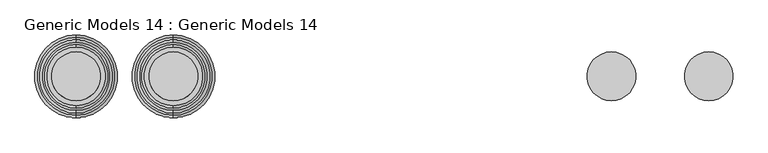
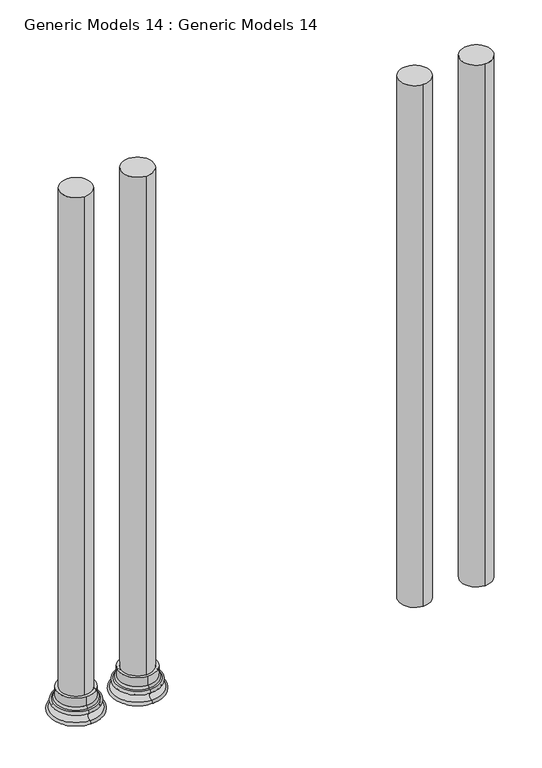
"""IFC4 building model written with IfcOpenShell, lengths in millimetres: proxy geometry, Generic Models 14 : Generic Models 14."""

from ifc_helpers import new_model, si_unit, point, frame, frame_2d, origin, place, context, project, spatial, polyline, circle_curve, ellipse_curve, trimmed, segment, composite_curve, outline, extrude, source, transform, mapped, element, save
from ifc_brep_helpers import plane_surface, cylinder_surface, revolved_surface, advanced_brep


def generic_models_14_generic_models_14_26f09abb(model_context):
    return source(origin(), model_context, "Body", "SolidModel", [
        advanced_brep(
        [(-2055.6825076, -7335.7292912, 330.2), (-2055.6825076, -7742.1292912, 330.2), (-2055.6825076, -7742.1292912, 304.8), (-2055.6825076, -7335.7292912, 304.8), (-2055.6825076, -7356.4126296, 381.908346), (-2055.6825076, -7721.4459527, 381.908346), (-2055.6825076, -7361.1292912, 406.4), (-2055.6825076, -7716.7292912, 406.4), (-2055.6825076, -7386.5292912, 431.8), (-2055.6825076, -7691.3292912, 431.8), (-2055.6825076, -7691.3292912, 406.4), (-2055.6825076, -7386.5292912, 406.4), (-2055.6825076, -7386.5292912, 508.0), (-2055.6825076, -7691.3292912, 508.0), (-2055.6825076, -7411.9292912, 304.8), (-2055.6825076, -7665.9292912, 304.8), (-2055.6825076, -7665.9292912, 508.0), (-2055.6825076, -7411.9292912, 508.0)],
        [
            (0, 1, circle_curve(frame((-2055.6825076, -7538.9292912, 330.2), z_axis=(0.0, 0.0, -1.0), x_axis=(0.0, -1.0, 0.0)), 203.2)),
            (1, 2, circle_curve(frame((-2055.6825076, -7742.1292912, 317.5), z_axis=(1.0, 0.0, 0.0), x_axis=(0.0, -1.0, 0.0)), 12.7)),
            (2, 3, circle_curve(frame((-2055.6825076, -7538.9292912, 304.8), z_axis=(0.0, 0.0, 1.0), x_axis=(0.0, -1.0, 0.0)), 203.2)),
            (3, 0, circle_curve(frame((-2055.6825076, -7335.7292912, 317.5), z_axis=(1.0, 0.0, 0.0), x_axis=(0.0, 1.0, 0.0)), 12.7)),
            (4, 5, circle_curve(frame((-2055.6825076, -7538.9292912, 381.908346), z_axis=(0.0, 0.0, -1.0), x_axis=(0.0, -1.0, 0.0)), 182.5166616)),
            (5, 1, circle_curve(frame((-2055.6825076, -7742.1292912, 360.1908407), z_axis=(-1.0, 0.0, 0.0), x_axis=(0.0, -1.0, 0.0)), 29.9908407)),
            (0, 4, circle_curve(frame((-2055.6825076, -7335.7292912, 360.1908407), z_axis=(-1.0, 0.0, 0.0), x_axis=(0.0, 1.0, 0.0)), 29.9908407)),
            (6, 7, circle_curve(frame((-2055.6825076, -7538.9292912, 406.4), z_axis=(0.0, 0.0, -1.0), x_axis=(0.0, -1.0, 0.0)), 177.8)),
            (7, 5, circle_curve(frame((-2055.6825076, -7716.7292912, 393.7), z_axis=(1.0, 0.0, 0.0), x_axis=(0.0, -1.0, 0.0)), 12.7)),
            (4, 6, circle_curve(frame((-2055.6825076, -7361.1292912, 393.7), z_axis=(1.0, 0.0, 0.0), x_axis=(0.0, 1.0, 0.0)), 12.7)),
            (8, 9, circle_curve(frame((-2055.6825076, -7538.9292912, 431.8), z_axis=(0.0, 0.0, -1.0), x_axis=(0.0, -1.0, 0.0)), 152.4)),
            (9, 10, circle_curve(frame((-2055.6825076, -7691.3292912, 419.1), z_axis=(1.0, 0.0, 0.0), x_axis=(0.0, -1.0, 0.0)), 12.7)),
            (10, 11, circle_curve(frame((-2055.6825076, -7538.9292912, 406.4), z_axis=(0.0, 0.0, 1.0), x_axis=(0.0, -1.0, 0.0)), 152.4)),
            (11, 8, circle_curve(frame((-2055.6825076, -7386.5292912, 419.1), z_axis=(1.0, 0.0, 0.0), x_axis=(0.0, 1.0, 0.0)), 12.7)),
            (12, 13, circle_curve(frame((-2055.6825076, -7538.9292912, 508.0), z_axis=(0.0, 0.0, -1.0), x_axis=(0.0, -1.0, 0.0)), 152.4)),
            (13, 9),
            (8, 12),
            (14, 15, circle_curve(frame((-2055.6825076, -7538.9292912, 304.8), z_axis=(0.0, 0.0, -1.0), x_axis=(0.0, -1.0, 0.0)), 127.0)),
            (15, 16),
            (16, 17, circle_curve(frame((-2055.6825076, -7538.9292912, 508.0), z_axis=(0.0, 0.0, 1.0), x_axis=(0.0, -1.0, 0.0)), 127.0)),
            (17, 14),
            (1, 0, circle_curve(frame((-2055.6825076, -7538.9292912, 330.2), z_axis=(0.0, 0.0, -1.0), x_axis=(0.0, 1.0, 0.0)), 203.2)),
            (3, 2, circle_curve(frame((-2055.6825076, -7538.9292912, 304.8), z_axis=(0.0, 0.0, 1.0), x_axis=(0.0, 1.0, 0.0)), 203.2)),
            (5, 4, circle_curve(frame((-2055.6825076, -7538.9292912, 381.908346), z_axis=(0.0, 0.0, -1.0), x_axis=(0.0, 1.0, 0.0)), 182.5166616)),
            (7, 6, circle_curve(frame((-2055.6825076, -7538.9292912, 406.4), z_axis=(0.0, 0.0, -1.0), x_axis=(0.0, 1.0, 0.0)), 177.8)),
            (10, 11, circle_curve(frame((-2055.6825076, -7538.9292912, 406.4), z_axis=(0.0, 0.0, -1.0), x_axis=(0.0, 1.0, 0.0)), 152.4)),
            (9, 8, circle_curve(frame((-2055.6825076, -7538.9292912, 431.8), z_axis=(0.0, 0.0, -1.0), x_axis=(0.0, 1.0, 0.0)), 152.4)),
            (13, 12, circle_curve(frame((-2055.6825076, -7538.9292912, 508.0), z_axis=(0.0, 0.0, -1.0), x_axis=(0.0, 1.0, 0.0)), 152.4)),
            (16, 17, circle_curve(frame((-2055.6825076, -7538.9292912, 508.0), z_axis=(0.0, 0.0, -1.0), x_axis=(0.0, 1.0, 0.0)), 127.0)),
            (15, 14, circle_curve(frame((-2055.6825076, -7538.9292912, 304.8), z_axis=(0.0, 0.0, -1.0), x_axis=(0.0, 1.0, 0.0)), 127.0)),
        ],
        [
            revolved_surface(trimmed(ellipse_curve(frame((-2055.6825076, -7742.1292912, 317.5), z_axis=(-1.0, 0.0, 0.0), x_axis=(0.0, -1.0, 0.0)), 12.7, 12.7), [point((-2055.6825076, -7742.1292912, 304.8))], [point((-2055.6825076, -7742.1292912, 330.2))], True, "CARTESIAN"), (-2055.6825076, -7538.9292912, 304.8), (0.0, 0.0, 1.0)),
            revolved_surface(trimmed(ellipse_curve(frame((-2055.6825076, -7742.1292912, 360.1908407), z_axis=(1.0, 0.0, 0.0), x_axis=(0.0, -1.0, 0.0)), 29.9908407, 29.9908407), [point((-2055.6825076, -7742.1292912, 330.2))], [point((-2055.6825076, -7721.4459527, 381.908346))], True, "CARTESIAN"), (-2055.6825076, -7538.9292912, 304.8), (0.0, 0.0, 1.0)),
            revolved_surface(trimmed(ellipse_curve(frame((-2055.6825076, -7716.7292912, 393.7), z_axis=(-1.0, 0.0, 0.0), x_axis=(0.0, -1.0, 0.0)), 12.7, 12.7), [point((-2055.6825076, -7721.4459527, 381.908346))], [point((-2055.6825076, -7716.7292912, 406.4))], True, "CARTESIAN"), (-2055.6825076, -7538.9292912, 304.8), (0.0, 0.0, 1.0)),
            revolved_surface(trimmed(ellipse_curve(frame((-2055.6825076, -7691.3292912, 419.1), z_axis=(-1.0, 0.0, 0.0), x_axis=(0.0, -1.0, 0.0)), 12.7, 12.7), [point((-2055.6825076, -7691.3292912, 406.4))], [point((-2055.6825076, -7691.3292912, 431.8))], True, "CARTESIAN"), (-2055.6825076, -7538.9292912, 304.8), (0.0, 0.0, 1.0)),
            cylinder_surface(frame((-2055.6825076, -7538.9292912, 304.8), z_axis=(0.0, 0.0, 1.0), x_axis=(0.0, -1.0, 0.0)), 152.4),
            revolved_surface(polyline([(-2055.6825076, -7665.9292912, 508.0), (-2055.6825076, -7665.9292912, 304.8)]), (-2055.6825076, -7538.9292912, 304.8), (0.0, 0.0, 1.0)),
            revolved_surface(trimmed(ellipse_curve(frame((-2055.6825076, -7335.7292912, 317.5), z_axis=(1.0, 0.0, 0.0), x_axis=(0.0, 1.0, 0.0)), 12.7, 12.7), [point((-2055.6825076, -7335.7292912, 304.8))], [point((-2055.6825076, -7335.7292912, 330.2))], True, "CARTESIAN"), (-2055.6825076, -7538.9292912, 304.8), (0.0, 0.0, 1.0)),
            revolved_surface(trimmed(ellipse_curve(frame((-2055.6825076, -7335.7292912, 360.1908407), z_axis=(-1.0, 0.0, 0.0), x_axis=(0.0, 1.0, 0.0)), 29.9908407, 29.9908407), [point((-2055.6825076, -7335.7292912, 330.2))], [point((-2055.6825076, -7356.4126296, 381.908346))], True, "CARTESIAN"), (-2055.6825076, -7538.9292912, 304.8), (0.0, 0.0, 1.0)),
            revolved_surface(trimmed(ellipse_curve(frame((-2055.6825076, -7361.1292912, 393.7), z_axis=(1.0, 0.0, 0.0), x_axis=(0.0, 1.0, 0.0)), 12.7, 12.7), [point((-2055.6825076, -7356.4126296, 381.908346))], [point((-2055.6825076, -7361.1292912, 406.4))], True, "CARTESIAN"), (-2055.6825076, -7538.9292912, 304.8), (0.0, 0.0, 1.0)),
            plane_surface(frame((-2055.6825076, -7538.9292912, 406.4), z_axis=(0.0, 0.0, 1.0), x_axis=(0.0, 1.0, 0.0))),
            revolved_surface(trimmed(ellipse_curve(frame((-2055.6825076, -7386.5292912, 419.1), z_axis=(1.0, 0.0, 0.0), x_axis=(0.0, 1.0, 0.0)), 12.7, 12.7), [point((-2055.6825076, -7386.5292912, 406.4))], [point((-2055.6825076, -7386.5292912, 431.8))], True, "CARTESIAN"), (-2055.6825076, -7538.9292912, 304.8), (0.0, 0.0, 1.0)),
            cylinder_surface(frame((-2055.6825076, -7538.9292912, 304.8), z_axis=(0.0, 0.0, 1.0), x_axis=(0.0, 1.0, 0.0)), 152.4),
            plane_surface(frame((-2055.6825076, -7538.9292912, 508.0), z_axis=(0.0, 0.0, 1.0), x_axis=(0.0, 1.0, 0.0))),
            revolved_surface(polyline([(-2055.6825076, -7411.9292912, 508.0), (-2055.6825076, -7411.9292912, 304.8)]), (-2055.6825076, -7538.9292912, 304.8), (0.0, 0.0, 1.0)),
            plane_surface(frame((-2055.6825076, -7538.9292912, 304.8), z_axis=(0.0, 0.0, -1.0), x_axis=(0.0, 1.0, 0.0))),
        ],
        [
            (0, [[1, 2, 3, 4]]),
            (1, [[5, 6, -1, 7]]),
            (2, [[8, 9, -5, 10]]),
            (3, [[11, 12, 13, 14]]),
            (4, [[15, 16, -11, 17]]),
            (5, [[18, 19, 20, 21]]),
            (6, [[22, -4, 23, -2]]),
            (7, [[24, -7, -22, -6]]),
            (8, [[25, -10, -24, -9]]),
            (9, [[-25, -8], [26, -13]]),
            (10, [[27, -14, -26, -12]]),
            (11, [[28, -17, -27, -16]]),
            (12, [[-28, -15], [29, -20]]),
            (13, [[30, -21, -29, -19]]),
            (14, [[-23, -3], [-30, -18]]),
        ],
    ),
        advanced_brep(
        [(-2563.6825076, -7335.7292912, 330.2), (-2563.6825076, -7742.1292912, 330.2), (-2563.6825076, -7742.1292912, 304.8), (-2563.6825076, -7335.7292912, 304.8), (-2563.6825076, -7356.4126296, 381.908346), (-2563.6825076, -7721.4459527, 381.908346), (-2563.6825076, -7361.1292912, 406.4), (-2563.6825076, -7716.7292912, 406.4), (-2563.6825076, -7386.5292912, 431.8), (-2563.6825076, -7691.3292912, 431.8), (-2563.6825076, -7691.3292912, 406.4), (-2563.6825076, -7386.5292912, 406.4), (-2563.6825076, -7386.5292912, 508.0), (-2563.6825076, -7691.3292912, 508.0), (-2563.6825076, -7411.9292912, 304.8), (-2563.6825076, -7665.9292912, 304.8), (-2563.6825076, -7665.9292912, 508.0), (-2563.6825076, -7411.9292912, 508.0)],
        [
            (0, 1, circle_curve(frame((-2563.6825076, -7538.9292912, 330.2), z_axis=(0.0, 0.0, -1.0), x_axis=(0.0, -1.0, 0.0)), 203.2)),
            (1, 2, circle_curve(frame((-2563.6825076, -7742.1292912, 317.5), z_axis=(1.0, 0.0, 0.0), x_axis=(0.0, -1.0, 0.0)), 12.7)),
            (2, 3, circle_curve(frame((-2563.6825076, -7538.9292912, 304.8), z_axis=(0.0, 0.0, 1.0), x_axis=(0.0, -1.0, 0.0)), 203.2)),
            (3, 0, circle_curve(frame((-2563.6825076, -7335.7292912, 317.5), z_axis=(1.0, 0.0, 0.0), x_axis=(0.0, 1.0, 0.0)), 12.7)),
            (4, 5, circle_curve(frame((-2563.6825076, -7538.9292912, 381.908346), z_axis=(0.0, 0.0, -1.0), x_axis=(0.0, -1.0, 0.0)), 182.5166616)),
            (5, 1, circle_curve(frame((-2563.6825076, -7742.1292912, 360.1908407), z_axis=(-1.0, 0.0, 0.0), x_axis=(0.0, -1.0, 0.0)), 29.9908407)),
            (0, 4, circle_curve(frame((-2563.6825076, -7335.7292912, 360.1908407), z_axis=(-1.0, 0.0, 0.0), x_axis=(0.0, 1.0, 0.0)), 29.9908407)),
            (6, 7, circle_curve(frame((-2563.6825076, -7538.9292912, 406.4), z_axis=(0.0, 0.0, -1.0), x_axis=(0.0, -1.0, 0.0)), 177.8)),
            (7, 5, circle_curve(frame((-2563.6825076, -7716.7292912, 393.7), z_axis=(1.0, 0.0, 0.0), x_axis=(0.0, -1.0, 0.0)), 12.7)),
            (4, 6, circle_curve(frame((-2563.6825076, -7361.1292912, 393.7), z_axis=(1.0, 0.0, 0.0), x_axis=(0.0, 1.0, 0.0)), 12.7)),
            (8, 9, circle_curve(frame((-2563.6825076, -7538.9292912, 431.8), z_axis=(0.0, 0.0, -1.0), x_axis=(0.0, -1.0, 0.0)), 152.4)),
            (9, 10, circle_curve(frame((-2563.6825076, -7691.3292912, 419.1), z_axis=(1.0, 0.0, 0.0), x_axis=(0.0, -1.0, 0.0)), 12.7)),
            (10, 11, circle_curve(frame((-2563.6825076, -7538.9292912, 406.4), z_axis=(0.0, 0.0, 1.0), x_axis=(0.0, -1.0, 0.0)), 152.4)),
            (11, 8, circle_curve(frame((-2563.6825076, -7386.5292912, 419.1), z_axis=(1.0, 0.0, 0.0), x_axis=(0.0, 1.0, 0.0)), 12.7)),
            (12, 13, circle_curve(frame((-2563.6825076, -7538.9292912, 508.0), z_axis=(0.0, 0.0, -1.0), x_axis=(0.0, -1.0, 0.0)), 152.4)),
            (13, 9),
            (8, 12),
            (14, 15, circle_curve(frame((-2563.6825076, -7538.9292912, 304.8), z_axis=(0.0, 0.0, -1.0), x_axis=(0.0, -1.0, 0.0)), 127.0)),
            (15, 16),
            (16, 17, circle_curve(frame((-2563.6825076, -7538.9292912, 508.0), z_axis=(0.0, 0.0, 1.0), x_axis=(0.0, -1.0, 0.0)), 127.0)),
            (17, 14),
            (1, 0, circle_curve(frame((-2563.6825076, -7538.9292912, 330.2), z_axis=(0.0, 0.0, -1.0), x_axis=(0.0, 1.0, 0.0)), 203.2)),
            (3, 2, circle_curve(frame((-2563.6825076, -7538.9292912, 304.8), z_axis=(0.0, 0.0, 1.0), x_axis=(0.0, 1.0, 0.0)), 203.2)),
            (5, 4, circle_curve(frame((-2563.6825076, -7538.9292912, 381.908346), z_axis=(0.0, 0.0, -1.0), x_axis=(0.0, 1.0, 0.0)), 182.5166616)),
            (7, 6, circle_curve(frame((-2563.6825076, -7538.9292912, 406.4), z_axis=(0.0, 0.0, -1.0), x_axis=(0.0, 1.0, 0.0)), 177.8)),
            (10, 11, circle_curve(frame((-2563.6825076, -7538.9292912, 406.4), z_axis=(0.0, 0.0, -1.0), x_axis=(0.0, 1.0, 0.0)), 152.4)),
            (9, 8, circle_curve(frame((-2563.6825076, -7538.9292912, 431.8), z_axis=(0.0, 0.0, -1.0), x_axis=(0.0, 1.0, 0.0)), 152.4)),
            (13, 12, circle_curve(frame((-2563.6825076, -7538.9292912, 508.0), z_axis=(0.0, 0.0, -1.0), x_axis=(0.0, 1.0, 0.0)), 152.4)),
            (16, 17, circle_curve(frame((-2563.6825076, -7538.9292912, 508.0), z_axis=(0.0, 0.0, -1.0), x_axis=(0.0, 1.0, 0.0)), 127.0)),
            (15, 14, circle_curve(frame((-2563.6825076, -7538.9292912, 304.8), z_axis=(0.0, 0.0, -1.0), x_axis=(0.0, 1.0, 0.0)), 127.0)),
        ],
        [
            revolved_surface(trimmed(ellipse_curve(frame((-2563.6825076, -7742.1292912, 317.5), z_axis=(-1.0, 0.0, 0.0), x_axis=(0.0, -1.0, 0.0)), 12.7, 12.7), [point((-2563.6825076, -7742.1292912, 304.8))], [point((-2563.6825076, -7742.1292912, 330.2))], True, "CARTESIAN"), (-2563.6825076, -7538.9292912, 304.8), (0.0, 0.0, 1.0)),
            revolved_surface(trimmed(ellipse_curve(frame((-2563.6825076, -7742.1292912, 360.1908407), z_axis=(1.0, 0.0, 0.0), x_axis=(0.0, -1.0, 0.0)), 29.9908407, 29.9908407), [point((-2563.6825076, -7742.1292912, 330.2))], [point((-2563.6825076, -7721.4459527, 381.908346))], True, "CARTESIAN"), (-2563.6825076, -7538.9292912, 304.8), (0.0, 0.0, 1.0)),
            revolved_surface(trimmed(ellipse_curve(frame((-2563.6825076, -7716.7292912, 393.7), z_axis=(-1.0, 0.0, 0.0), x_axis=(0.0, -1.0, 0.0)), 12.7, 12.7), [point((-2563.6825076, -7721.4459527, 381.908346))], [point((-2563.6825076, -7716.7292912, 406.4))], True, "CARTESIAN"), (-2563.6825076, -7538.9292912, 304.8), (0.0, 0.0, 1.0)),
            revolved_surface(trimmed(ellipse_curve(frame((-2563.6825076, -7691.3292912, 419.1), z_axis=(-1.0, 0.0, 0.0), x_axis=(0.0, -1.0, 0.0)), 12.7, 12.7), [point((-2563.6825076, -7691.3292912, 406.4))], [point((-2563.6825076, -7691.3292912, 431.8))], True, "CARTESIAN"), (-2563.6825076, -7538.9292912, 304.8), (0.0, 0.0, 1.0)),
            cylinder_surface(frame((-2563.6825076, -7538.9292912, 304.8), z_axis=(0.0, 0.0, 1.0), x_axis=(0.0, -1.0, 0.0)), 152.4),
            revolved_surface(polyline([(-2563.6825076, -7665.9292912, 508.0), (-2563.6825076, -7665.9292912, 304.8)]), (-2563.6825076, -7538.9292912, 304.8), (0.0, 0.0, 1.0)),
            revolved_surface(trimmed(ellipse_curve(frame((-2563.6825076, -7335.7292912, 317.5), z_axis=(1.0, 0.0, 0.0), x_axis=(0.0, 1.0, 0.0)), 12.7, 12.7), [point((-2563.6825076, -7335.7292912, 304.8))], [point((-2563.6825076, -7335.7292912, 330.2))], True, "CARTESIAN"), (-2563.6825076, -7538.9292912, 304.8), (0.0, 0.0, 1.0)),
            revolved_surface(trimmed(ellipse_curve(frame((-2563.6825076, -7335.7292912, 360.1908407), z_axis=(-1.0, 0.0, 0.0), x_axis=(0.0, 1.0, 0.0)), 29.9908407, 29.9908407), [point((-2563.6825076, -7335.7292912, 330.2))], [point((-2563.6825076, -7356.4126296, 381.908346))], True, "CARTESIAN"), (-2563.6825076, -7538.9292912, 304.8), (0.0, 0.0, 1.0)),
            revolved_surface(trimmed(ellipse_curve(frame((-2563.6825076, -7361.1292912, 393.7), z_axis=(1.0, 0.0, 0.0), x_axis=(0.0, 1.0, 0.0)), 12.7, 12.7), [point((-2563.6825076, -7356.4126296, 381.908346))], [point((-2563.6825076, -7361.1292912, 406.4))], True, "CARTESIAN"), (-2563.6825076, -7538.9292912, 304.8), (0.0, 0.0, 1.0)),
            plane_surface(frame((-2563.6825076, -7538.9292912, 406.4), z_axis=(0.0, 0.0, 1.0), x_axis=(0.0, 1.0, 0.0))),
            revolved_surface(trimmed(ellipse_curve(frame((-2563.6825076, -7386.5292912, 419.1), z_axis=(1.0, 0.0, 0.0), x_axis=(0.0, 1.0, 0.0)), 12.7, 12.7), [point((-2563.6825076, -7386.5292912, 406.4))], [point((-2563.6825076, -7386.5292912, 431.8))], True, "CARTESIAN"), (-2563.6825076, -7538.9292912, 304.8), (0.0, 0.0, 1.0)),
            cylinder_surface(frame((-2563.6825076, -7538.9292912, 304.8), z_axis=(0.0, 0.0, 1.0), x_axis=(0.0, 1.0, 0.0)), 152.4),
            plane_surface(frame((-2563.6825076, -7538.9292912, 508.0), z_axis=(0.0, 0.0, 1.0), x_axis=(0.0, 1.0, 0.0))),
            revolved_surface(polyline([(-2563.6825076, -7411.9292912, 508.0), (-2563.6825076, -7411.9292912, 304.8)]), (-2563.6825076, -7538.9292912, 304.8), (0.0, 0.0, 1.0)),
            plane_surface(frame((-2563.6825076, -7538.9292912, 304.8), z_axis=(0.0, 0.0, -1.0), x_axis=(0.0, 1.0, 0.0))),
        ],
        [
            (0, [[1, 2, 3, 4]]),
            (1, [[5, 6, -1, 7]]),
            (2, [[8, 9, -5, 10]]),
            (3, [[11, 12, 13, 14]]),
            (4, [[15, 16, -11, 17]]),
            (5, [[18, 19, 20, 21]]),
            (6, [[22, -4, 23, -2]]),
            (7, [[24, -7, -22, -6]]),
            (8, [[25, -10, -24, -9]]),
            (9, [[-25, -8], [26, -13]]),
            (10, [[27, -14, -26, -12]]),
            (11, [[28, -17, -27, -16]]),
            (12, [[-28, -15], [29, -20]]),
            (13, [[30, -21, -29, -19]]),
            (14, [[-23, -3], [-30, -18]]),
        ],
    ),
        extrude(outline(composite_curve([segment(trimmed(circle_curve(frame_2d((-2563.6825076, -7538.9292912)), 127.0), [point((-2563.6825076, -7665.9292912))], [point((-2563.6825076, -7411.9292912))], False, "CARTESIAN"), True, "CONTINUOUS"), segment(trimmed(circle_curve(frame_2d((-2563.6825076, -7538.9292912)), 127.0), [point((-2563.6825076, -7411.9292912))], [point((-2563.6825076, -7665.9292912))], False, "CARTESIAN"), True, "CONTINUOUS")], self_intersect=False)), frame((0.0, 0.0, 304.8), z_axis=(0.0, 0.0, 1.0), x_axis=(1.0, 0.0, 0.0)), (0.0, 0.0, 1.0), 4546.6),
        extrude(outline(composite_curve([segment(trimmed(circle_curve(frame_2d((-2055.6825076, -7538.9292912)), 127.0), [point((-2055.6825076, -7665.9292912))], [point((-2055.6825076, -7411.9292912))], False, "CARTESIAN"), True, "CONTINUOUS"), segment(trimmed(circle_curve(frame_2d((-2055.6825076, -7538.9292912)), 127.0), [point((-2055.6825076, -7411.9292912))], [point((-2055.6825076, -7665.9292912))], False, "CARTESIAN"), True, "CONTINUOUS")], self_intersect=False)), frame((0.0, 0.0, 304.8), z_axis=(0.0, 0.0, 1.0), x_axis=(1.0, 0.0, 0.0)), (0.0, 0.0, 1.0), 4546.6),
        extrude(outline(composite_curve([segment(trimmed(circle_curve(frame_2d((738.3174924, -7538.9292912)), 127.0), [point((738.3174924, -7665.9292912))], [point((738.3174924, -7411.9292912))], False, "CARTESIAN"), True, "CONTINUOUS"), segment(trimmed(circle_curve(frame_2d((738.3174924, -7538.9292912)), 127.0), [point((738.3174924, -7411.9292912))], [point((738.3174924, -7665.9292912))], False, "CARTESIAN"), True, "CONTINUOUS")], self_intersect=False)), frame((0.0, 0.0, 304.8), z_axis=(0.0, 0.0, 1.0), x_axis=(1.0, 0.0, 0.0)), (0.0, 0.0, 1.0), 4546.6),
        extrude(outline(composite_curve([segment(trimmed(circle_curve(frame_2d((230.3174924, -7538.9292912)), 127.0), [point((230.3174924, -7665.9292912))], [point((230.3174924, -7411.9292912))], False, "CARTESIAN"), True, "CONTINUOUS"), segment(trimmed(circle_curve(frame_2d((230.3174924, -7538.9292912)), 127.0), [point((230.3174924, -7411.9292912))], [point((230.3174924, -7665.9292912))], False, "CARTESIAN"), True, "CONTINUOUS")], self_intersect=False)), frame((0.0, 0.0, 304.8), z_axis=(0.0, 0.0, 1.0), x_axis=(1.0, 0.0, 0.0)), (0.0, 0.0, 1.0), 4546.6),
    ])


if __name__ == "__main__":
    model = new_model("IFC4")
    model_context = context("Model", 3, world=origin())
    ifc_project = project(units=[si_unit("LENGTHUNIT", "METRE", prefix="MILLI")], contexts=[model_context])
    site = spatial("IfcSite", under=ifc_project)
    building = spatial("IfcBuilding", under=site)
    placement = place(None, origin())
    generic_models_14_generic_models_14_shape = generic_models_14_generic_models_14_26f09abb(model_context)
    element("IfcBuildingElementProxy", 1, Name="Generic Models 14 : Generic Models 14", ObjectType="Generic Models 14 : Generic Models 14", at=placement, inside=building, context=model_context, shape_type="MappedRepresentation", body=[
        mapped(generic_models_14_generic_models_14_shape, transform((0.0, 0.0, 0.0), x_axis=(1.0, 0.0, 0.0), y_axis=(0.0, 1.0, 0.0), z_axis=(0.0, 0.0, 1.0))),
    ])
    save(model, "model.ifc")
